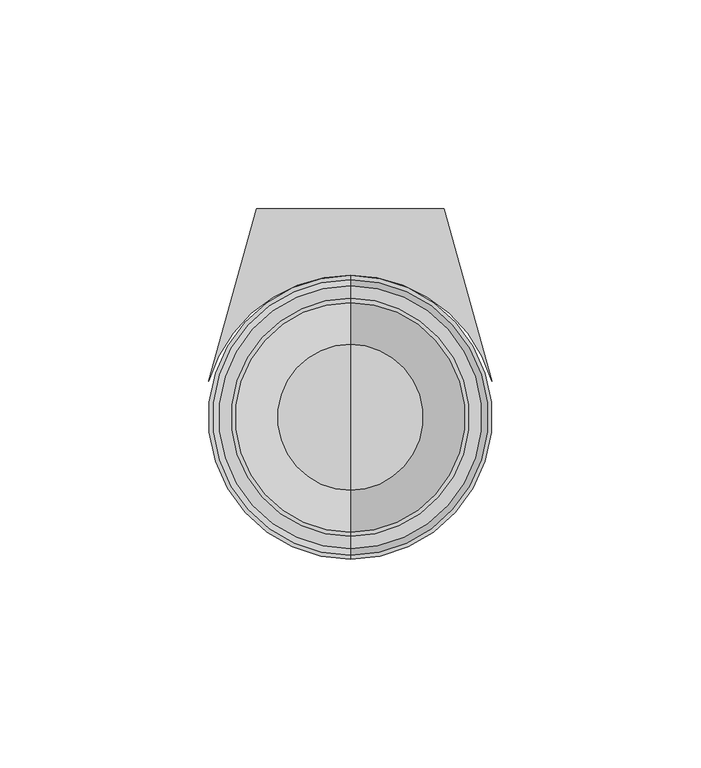
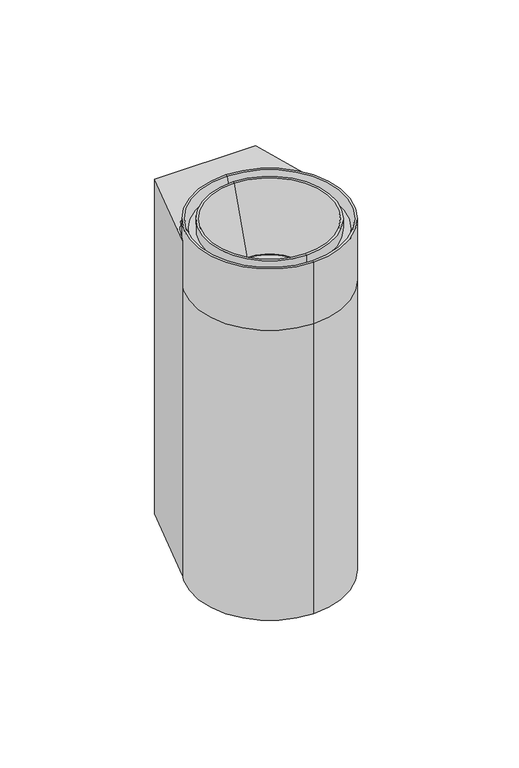
"""IFC4 building model written with IfcOpenShell, lengths in millimetres: light fixture geometry."""

from ifc_helpers import new_model, si_unit, point, frame, frame_2d, origin, place, context, project, spatial, polyline, circle_curve, trimmed, segment, composite_curve, outline, extrude, source, transform, mapped, element, save
from ifc_brep_helpers import plane_surface, cylinder_surface, revolved_surface, advanced_brep


def light_fixture_d13112ec(model_context):
    return source(origin(), model_context, "Body", "SolidModel", [
        extrude(outline(composite_curve([segment(polyline([(22.5, 0.0), (34.0, -41.4)]), True, "CONTINUOUS"), segment(trimmed(circle_curve(frame_2d((0.1055807, -51.314577)), 35.3147348), [point((34.0, -41.4))], [point((0.0, -16.0))], True, "CARTESIAN"), True, "CONTINUOUS"), segment(trimmed(circle_curve(frame_2d((-0.1055807, -51.314577)), 35.3147348), [point((0.0, -16.0))], [point((-34.0, -41.4))], True, "CARTESIAN"), True, "CONTINUOUS"), segment(polyline([(-34.0, -41.4), (-22.5, 0.0), (22.5, 0.0)]), True, "CONTINUOUS")], self_intersect=False)), frame((0.0, 0.0, -79.0), z_axis=(0.0, 0.0, 1.0), x_axis=(1.0, 0.0, 0.0)), (0.0, 0.0, 1.0), 158.1703709),
        advanced_brep(
        [(0.0, -16.0, 54.0), (0.0, -84.0, 54.0), (0.0, -84.0, 83.0), (0.0, -16.0, 83.0), (0.0, -16.0, -83.0), (0.0, -84.0, -83.0), (0.0, -17.0, -83.0), (0.0, -83.0, -83.0), (0.0, -18.5, -78.0), (0.0, -81.5, -78.0), (0.0, -21.5, -78.0), (0.0, -78.5, -78.0), (0.0, -21.5, -83.0), (0.0, -78.5, -83.0), (0.0, -22.5, -83.0), (0.0, -77.5, -83.0), (0.0, -32.5, -54.0), (0.0, -67.5, -54.0), (0.0, -32.5, -52.0), (0.0, -67.5, -52.0), (0.0, -32.5, 54.0), (0.0, -67.5, 54.0), (0.0, -22.5, 83.0), (0.0, -77.5, 83.0), (0.0, -21.5, 83.0), (0.0, -78.5, 83.0), (0.0, -21.5, 78.0), (0.0, -78.5, 78.0), (0.0, -18.5, 78.0), (0.0, -81.5, 78.0), (0.0, -17.0, 83.0), (0.0, -83.0, 83.0)],
        [
            (0, 1, circle_curve(frame((0.0, -50.0, 54.0), z_axis=(0.0, 0.0, 1.0), x_axis=(0.0, -1.0, 0.0)), 34.0)),
            (1, 2),
            (2, 3, circle_curve(frame((0.0, -50.0, 83.0), z_axis=(0.0, 0.0, -1.0), x_axis=(0.0, -1.0, 0.0)), 34.0)),
            (3, 0),
            (1, 0, circle_curve(frame((0.0, -50.0, 54.0), z_axis=(0.0, 0.0, 1.0), x_axis=(0.0, -1.0, 0.0)), 34.0)),
            (3, 2, circle_curve(frame((0.0, -50.0, 83.0), z_axis=(0.0, 0.0, -1.0), x_axis=(0.0, -1.0, 0.0)), 34.0)),
            (4, 5, circle_curve(frame((0.0, -50.0, -83.0), z_axis=(0.0, 0.0, 1.0), x_axis=(0.0, -1.0, 0.0)), 34.0)),
            (5, 1),
            (0, 4),
            (5, 4, circle_curve(frame((0.0, -50.0, -83.0), z_axis=(0.0, 0.0, 1.0), x_axis=(0.0, -1.0, 0.0)), 34.0)),
            (6, 7, circle_curve(frame((0.0, -50.0, -83.0), z_axis=(0.0, 0.0, 1.0), x_axis=(0.0, -1.0, 0.0)), 33.0)),
            (7, 5),
            (4, 6),
            (7, 6, circle_curve(frame((0.0, -50.0, -83.0), z_axis=(0.0, 0.0, 1.0), x_axis=(0.0, -1.0, 0.0)), 33.0)),
            (8, 9, circle_curve(frame((0.0, -50.0, -78.0), z_axis=(0.0, 0.0, 1.0), x_axis=(0.0, -1.0, 0.0)), 31.5)),
            (9, 7),
            (6, 8),
            (9, 8, circle_curve(frame((0.0, -50.0, -78.0), z_axis=(0.0, 0.0, 1.0), x_axis=(0.0, -1.0, 0.0)), 31.5)),
            (10, 11, circle_curve(frame((0.0, -50.0, -78.0), z_axis=(0.0, 0.0, 1.0), x_axis=(0.0, -1.0, 0.0)), 28.5)),
            (11, 9),
            (8, 10),
            (11, 10, circle_curve(frame((0.0, -50.0, -78.0), z_axis=(0.0, 0.0, 1.0), x_axis=(0.0, -1.0, 0.0)), 28.5)),
            (12, 13, circle_curve(frame((0.0, -50.0, -83.0), z_axis=(0.0, 0.0, 1.0), x_axis=(0.0, -1.0, 0.0)), 28.5)),
            (13, 11),
            (10, 12),
            (13, 12, circle_curve(frame((0.0, -50.0, -83.0), z_axis=(0.0, 0.0, 1.0), x_axis=(0.0, -1.0, 0.0)), 28.5)),
            (14, 15, circle_curve(frame((0.0, -50.0, -83.0), z_axis=(0.0, 0.0, 1.0), x_axis=(0.0, -1.0, 0.0)), 27.5)),
            (15, 13),
            (12, 14),
            (15, 14, circle_curve(frame((0.0, -50.0, -83.0), z_axis=(0.0, 0.0, 1.0), x_axis=(0.0, -1.0, 0.0)), 27.5)),
            (16, 17, circle_curve(frame((0.0, -50.0, -54.0), z_axis=(0.0, 0.0, 1.0), x_axis=(0.0, -1.0, 0.0)), 17.5)),
            (17, 15),
            (14, 16),
            (17, 16, circle_curve(frame((0.0, -50.0, -54.0), z_axis=(0.0, 0.0, 1.0), x_axis=(0.0, -1.0, 0.0)), 17.5)),
            (18, 19, circle_curve(frame((0.0, -50.0, -52.0), z_axis=(0.0, 0.0, 1.0), x_axis=(0.0, -1.0, 0.0)), 17.5)),
            (19, 17),
            (16, 18),
            (19, 18, circle_curve(frame((0.0, -50.0, -52.0), z_axis=(0.0, 0.0, 1.0), x_axis=(0.0, -1.0, 0.0)), 17.5)),
            (20, 21, circle_curve(frame((0.0, -50.0, 54.0), z_axis=(0.0, 0.0, 1.0), x_axis=(0.0, -1.0, 0.0)), 17.5)),
            (21, 19),
            (18, 20),
            (21, 20, circle_curve(frame((0.0, -50.0, 54.0), z_axis=(0.0, 0.0, 1.0), x_axis=(0.0, -1.0, 0.0)), 17.5)),
            (22, 23, circle_curve(frame((0.0, -50.0, 83.0), z_axis=(0.0, 0.0, 1.0), x_axis=(0.0, -1.0, 0.0)), 27.5)),
            (23, 21),
            (20, 22),
            (23, 22, circle_curve(frame((0.0, -50.0, 83.0), z_axis=(0.0, 0.0, 1.0), x_axis=(0.0, -1.0, 0.0)), 27.5)),
            (24, 25, circle_curve(frame((0.0, -50.0, 83.0), z_axis=(0.0, 0.0, 1.0), x_axis=(0.0, -1.0, 0.0)), 28.5)),
            (25, 23),
            (22, 24),
            (25, 24, circle_curve(frame((0.0, -50.0, 83.0), z_axis=(0.0, 0.0, 1.0), x_axis=(0.0, -1.0, 0.0)), 28.5)),
            (26, 27, circle_curve(frame((0.0, -50.0, 78.0), z_axis=(0.0, 0.0, 1.0), x_axis=(0.0, -1.0, 0.0)), 28.5)),
            (27, 25),
            (24, 26),
            (27, 26, circle_curve(frame((0.0, -50.0, 78.0), z_axis=(0.0, 0.0, 1.0), x_axis=(0.0, -1.0, 0.0)), 28.5)),
            (28, 29, circle_curve(frame((0.0, -50.0, 78.0), z_axis=(0.0, 0.0, 1.0), x_axis=(0.0, -1.0, 0.0)), 31.5)),
            (29, 27),
            (26, 28),
            (29, 28, circle_curve(frame((0.0, -50.0, 78.0), z_axis=(0.0, 0.0, 1.0), x_axis=(0.0, -1.0, 0.0)), 31.5)),
            (30, 31, circle_curve(frame((0.0, -50.0, 83.0), z_axis=(0.0, 0.0, 1.0), x_axis=(0.0, -1.0, 0.0)), 33.0)),
            (31, 29),
            (28, 30),
            (31, 30, circle_curve(frame((0.0, -50.0, 83.0), z_axis=(0.0, 0.0, 1.0), x_axis=(0.0, -1.0, 0.0)), 33.0)),
            (2, 31),
            (30, 3),
        ],
        [
            cylinder_surface(frame((0.0, -50.0, -744.5420944), z_axis=(0.0, 0.0, -1.0), x_axis=(0.0, -1.0, 0.0)), 34.0),
            plane_surface(frame((0.0, -50.0, -83.0), z_axis=(0.0, 0.0, -1.0), x_axis=(0.0, -1.0, 0.0))),
            revolved_surface(polyline([(0.0, -83.0, -83.0), (0.0, -81.5, -78.0)]), (0.0, -50.0, -744.5420944), (0.0, 0.0, -1.0)),
            plane_surface(frame((0.0, -50.0, -78.0), z_axis=(0.0, 0.0, -1.0), x_axis=(0.0, -1.0, 0.0))),
            cylinder_surface(frame((0.0, -50.0, -744.5420944), z_axis=(0.0, 0.0, -1.0), x_axis=(0.0, -1.0, 0.0)), 28.5),
            revolved_surface(polyline([(0.0, -77.5, -83.0), (0.0, -67.5, -54.0)]), (0.0, -50.0, -744.5420944), (0.0, 0.0, -1.0)),
            revolved_surface(polyline([(0.0, -67.5, -54.0), (0.0, -67.5, -52.0)]), (0.0, -50.0, -744.5420944), (0.0, 0.0, -1.0)),
            revolved_surface(polyline([(0.0, -67.5, -52.0), (0.0, -67.5, 54.0)]), (0.0, -50.0, -744.5420944), (0.0, 0.0, -1.0)),
            revolved_surface(polyline([(0.0, -67.5, 54.0), (0.0, -77.5, 83.0)]), (0.0, -50.0, -744.5420944), (0.0, 0.0, -1.0)),
            plane_surface(frame((0.0, -50.0, 83.0), z_axis=(0.0, 0.0, 1.0), x_axis=(0.0, -1.0, 0.0))),
            plane_surface(frame((0.0, -50.0, 78.0), z_axis=(0.0, 0.0, 1.0), x_axis=(0.0, -1.0, 0.0))),
            revolved_surface(polyline([(0.0, -81.5, 78.0), (0.0, -83.0, 83.0)]), (0.0, -50.0, -744.5420944), (0.0, 0.0, -1.0)),
        ],
        [
            (0, [[1, 2, 3, 4]]),
            (0, [[5, -4, 6, -2]]),
            (0, [[7, 8, -1, 9]]),
            (0, [[10, -9, -5, -8]]),
            (1, [[11, 12, -7, 13]]),
            (1, [[14, -13, -10, -12]]),
            (2, [[15, 16, -11, 17]]),
            (2, [[18, -17, -14, -16]]),
            (3, [[19, 20, -15, 21]]),
            (3, [[22, -21, -18, -20]]),
            (4, [[23, 24, -19, 25]]),
            (4, [[26, -25, -22, -24]]),
            (1, [[27, 28, -23, 29]]),
            (1, [[30, -29, -26, -28]]),
            (5, [[31, 32, -27, 33]]),
            (5, [[34, -33, -30, -32]]),
            (6, [[35, 36, -31, 37]]),
            (6, [[38, -37, -34, -36]]),
            (7, [[39, 40, -35, 41]]),
            (7, [[42, -41, -38, -40]]),
            (8, [[43, 44, -39, 45]]),
            (8, [[46, -45, -42, -44]]),
            (9, [[47, 48, -43, 49]]),
            (9, [[50, -49, -46, -48]]),
            (4, [[51, 52, -47, 53]]),
            (4, [[54, -53, -50, -52]]),
            (10, [[55, 56, -51, 57]]),
            (10, [[58, -57, -54, -56]]),
            (11, [[59, 60, -55, 61]]),
            (11, [[62, -61, -58, -60]]),
            (9, [[-3, 63, -59, 64]]),
            (9, [[-6, -64, -62, -63]]),
        ],
    ),
        advanced_brep(
        [(0.0, -32.5, -52.0), (0.0, -67.5, -52.0), (0.0, -50.0, -52.0), (0.0, -32.5, -54.0), (0.0, -67.5, -54.0), (0.0, -50.0, -54.0)],
        [
            (0, 1, circle_curve(frame((0.0, -50.0, -52.0), z_axis=(0.0, 0.0, 1.0), x_axis=(0.0, -1.0, 0.0)), 17.5)),
            (1, 2),
            (2, 0),
            (1, 0, circle_curve(frame((0.0, -50.0, -52.0), z_axis=(0.0, 0.0, 1.0), x_axis=(0.0, -1.0, 0.0)), 17.5)),
            (3, 4, circle_curve(frame((0.0, -50.0, -54.0), z_axis=(0.0, 0.0, 1.0), x_axis=(0.0, -1.0, 0.0)), 17.5)),
            (4, 1),
            (0, 3),
            (4, 3, circle_curve(frame((0.0, -50.0, -54.0), z_axis=(0.0, 0.0, 1.0), x_axis=(0.0, -1.0, 0.0)), 17.5)),
            (5, 4),
            (3, 5),
        ],
        [
            plane_surface(frame((0.0, -50.0, -52.0), z_axis=(0.0, 0.0, 1.0), x_axis=(0.0, -1.0, 0.0))),
            cylinder_surface(frame((0.0, -50.0, -816.5420944), z_axis=(0.0, 0.0, -1.0), x_axis=(0.0, -1.0, 0.0)), 17.5),
            plane_surface(frame((0.0, -50.0, -54.0), z_axis=(0.0, 0.0, -1.0), x_axis=(0.0, -1.0, 0.0))),
        ],
        [
            (0, [[1, 2, 3]]),
            (0, [[4, -3, -2]]),
            (1, [[5, 6, -1, 7]]),
            (1, [[8, -7, -4, -6]]),
            (2, [[9, -5, 10]]),
            (2, [[-10, -8, -9]]),
        ],
    ),
        advanced_brep(
        [(0.0, -32.5, 54.0), (0.0, -67.5, 54.0), (0.0, -50.0, 54.0), (0.0, -32.5, 52.0), (0.0, -67.5, 52.0), (0.0, -50.0, 52.0)],
        [
            (0, 1, circle_curve(frame((0.0, -50.0, 54.0), z_axis=(0.0, 0.0, 1.0), x_axis=(0.0, -1.0, 0.0)), 17.5)),
            (1, 2),
            (2, 0),
            (1, 0, circle_curve(frame((0.0, -50.0, 54.0), z_axis=(0.0, 0.0, 1.0), x_axis=(0.0, -1.0, 0.0)), 17.5)),
            (3, 4, circle_curve(frame((0.0, -50.0, 52.0), z_axis=(0.0, 0.0, 1.0), x_axis=(0.0, -1.0, 0.0)), 17.5)),
            (4, 1),
            (0, 3),
            (4, 3, circle_curve(frame((0.0, -50.0, 52.0), z_axis=(0.0, 0.0, 1.0), x_axis=(0.0, -1.0, 0.0)), 17.5)),
            (5, 4),
            (3, 5),
        ],
        [
            plane_surface(frame((0.0, -50.0, 54.0), z_axis=(0.0, 0.0, 1.0), x_axis=(0.0, -1.0, 0.0))),
            cylinder_surface(frame((0.0, -50.0, -710.5420944), z_axis=(0.0, 0.0, -1.0), x_axis=(0.0, -1.0, 0.0)), 17.5),
            plane_surface(frame((0.0, -50.0, 52.0), z_axis=(0.0, 0.0, -1.0), x_axis=(0.0, -1.0, 0.0))),
        ],
        [
            (0, [[1, 2, 3]]),
            (0, [[4, -3, -2]]),
            (1, [[5, 6, -1, 7]]),
            (1, [[8, -7, -4, -6]]),
            (2, [[9, -5, 10]]),
            (2, [[-10, -8, -9]]),
        ],
    ),
    ])


if __name__ == "__main__":
    model = new_model("IFC4")
    model_context = context("Model", 3, world=origin())
    ifc_project = project(units=[si_unit("LENGTHUNIT", "METRE", prefix="MILLI")], contexts=[model_context])
    site = spatial("IfcSite", under=ifc_project)
    building = spatial("IfcBuilding", under=site)
    placement = place(None, origin())
    light_fixture_shape = light_fixture_d13112ec(model_context)
    element("IfcLightFixture", 1, at=placement, inside=building, context=model_context, shape_type="MappedRepresentation", body=[
        mapped(light_fixture_shape, transform((0.0, 0.0, 0.0), x_axis=(1.0, 0.0, 0.0), y_axis=(0.0, 1.0, 0.0), z_axis=(0.0, 0.0, 1.0))),
    ])
    save(model, "model.ifc")

# Revit data of these elements
# Type
#   URL = "https://products-archive.xal.com/product/xal/048-31604111O"
#   Type Tag = ""
#   System = ""
#   Sorting Reference = ""
#   Schedule ID = "1"
#   Product Info = "SASSO 60 round direct / indirect wall | jet black | 2700 K | non DIM | UGR ?  22 | 1170 lm"
#   Photometric Web File = "XAL-OPAL-LAMBERTSCH_F16_AD62946.ies"
#   Optic = "opal (lambertsch)"
#   Manufacturer = "XAL"
#   Luminous Flux = "1170"
#   Item Number = "048-31604111O"
#   Initial Color Temperature = "2700 K"
#   Housing Color = "black/black"
#   Glare Rating = "22"
#   Description = "Cylindrical wall surface mounted luminaire made of aluminium; surface jet black powder coated;  passive cooling of the LEDs through improved heat sink geometry; with COB (Chip on Board) technology for maximum efficiency; no appearance of multiple shadows; light color 2700 K;  energy efficient LEDs with high CRI; incl. high quality lens system; homogeneous wall or ceiling illumination through uniform light distribution; direct/indirect light distribution;    incl. converter, non dimmable;  \r\nGeneral: jet black, 1170 lm\r\nLED: 2700 K\r\nOptical: opal (lambertsch), UGR ? 22\r\nElectrical: non DIM,  system 20.6 W\r\nPhysical: length 68 mm, width 84 mm, height 166 mm"
#   Control = "non DIM"
#   Color Temperature = "2700 K"
#   Catalog Number = "048-31604111O"
#   Assembly ID [instance] = ""
#   Additional Reference [instance] = ""
#   W = 0' - 3.30709"
#   Type Tag Object Distance [instance] = 0' - 0"
#   Type Tag Distance [instance] = 0' - 9.84252"
#   Type Tag Base Position [instance] = 0' - 9.84252"
#   Power = 20.6 W
#   L = 0' - 2.67717"
#   H = 0' - 6.53543"
#   Emit from Width = 1' - 3.74803"
#   Emit from Length = 0' - 3.93701"
#   Emit from Diameter = 0' - 2.16535"
#   Default Elevation = 4' - 0"
#   Type Tag Upper Position [instance] = no
#   Type Tag On [instance] = no
#   Type Tag Lower Position [instance] = yes
#   Tag Frame [instance] = no
#   Pcs. per Package = 1
#   Tag Size = element 383008
#   Product Color Secondary = XAL_JET_BLACK
#   Product Color Primary = XAL_JET_BLACK
#   Light type = element 382996
# Element 1 (IfcLightFixture)
#   Materials on its faces: "XAL_JET_BLACK", "XAL_DIFFUSE"
# Materials
#   "XAL_JET_BLACK": class "Metal", colour RGB 82 82 82, transparency 0, Description = "Steel, Matte structure coat", Cost = 0
#   "XAL_DIFFUSE": class "Plastic", colour RGB 255 255 255, transparency 0, Manufacturer = "XAL", Description = "PMMA MATERIAL OPAL 3000K", Cost = 0
